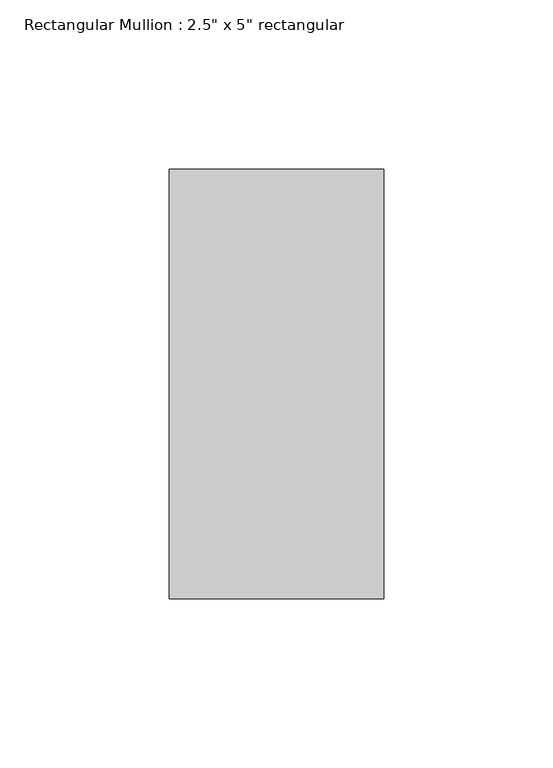
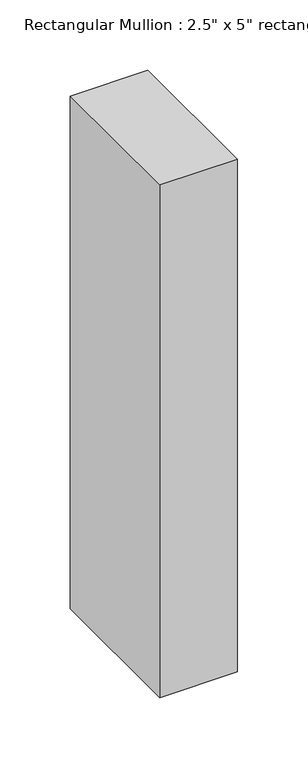
"""IFC4 building model written with IfcOpenShell, lengths in millimetres: member geometry."""

from ifc_helpers import new_model, si_unit, frame, origin, place, context, project, spatial, polyline, outline, extrude, source, transform, mapped, element, save


def member_56ec01f9(model_context):
    return source(origin(), model_context, "Body", "SweptSolid", [
        extrude(outline(polyline([(0.0, 63.5), (0.0, -63.5), (-63.5, -63.5), (-63.5, 63.5), (0.0, 63.5)])), frame((0.0, 0.0, -444.7313568), z_axis=(0.0, 0.0, 1.0), x_axis=(1.0, 0.0, 0.0)), (0.0, 0.0, 1.0), 444.7313568),
    ])


if __name__ == "__main__":
    model = new_model("IFC4")
    model_context = context("Model", 3, world=origin())
    ifc_project = project(units=[si_unit("LENGTHUNIT", "METRE", prefix="MILLI")], contexts=[model_context])
    site = spatial("IfcSite", under=ifc_project)
    building = spatial("IfcBuilding", under=site)
    placement = place(None, origin())
    member_shape = member_56ec01f9(model_context)
    element("IfcMember", 1, ObjectType="Rectangular Mullion : 2.5\" x 5\" rectangular", at=placement, inside=building, context=model_context, shape_type="MappedRepresentation", body=[
        mapped(member_shape, transform((0.0, 0.0, 0.0), x_axis=(1.0, 0.0, 0.0), y_axis=(0.0, 1.0, 0.0), z_axis=(0.0, 0.0, 1.0))),
    ])
    save(model, "model.ifc")

# Revit data of these elements
# Type "Rectangular Mullion : 2.5\" x 5\" rectangular"
#   built-in parameter 1007304 = 0.416667 (stored number, unit not read)
#   built-in parameter 1007301 = 0.104167 (stored number, unit not read)
#   built-in parameter 1007300 = 0.104167 (stored number, unit not read)
# Element 1 (IfcMember, "Rectangular Mullion : 2.5\" x 5\" rectangular")
#   Materials on its faces: "Aluminum"
# Materials
#   "Aluminum": class "Metal", colour RGB 247 247 247, transparency 0, Description = "Aluminum 6061", Cost = 0
